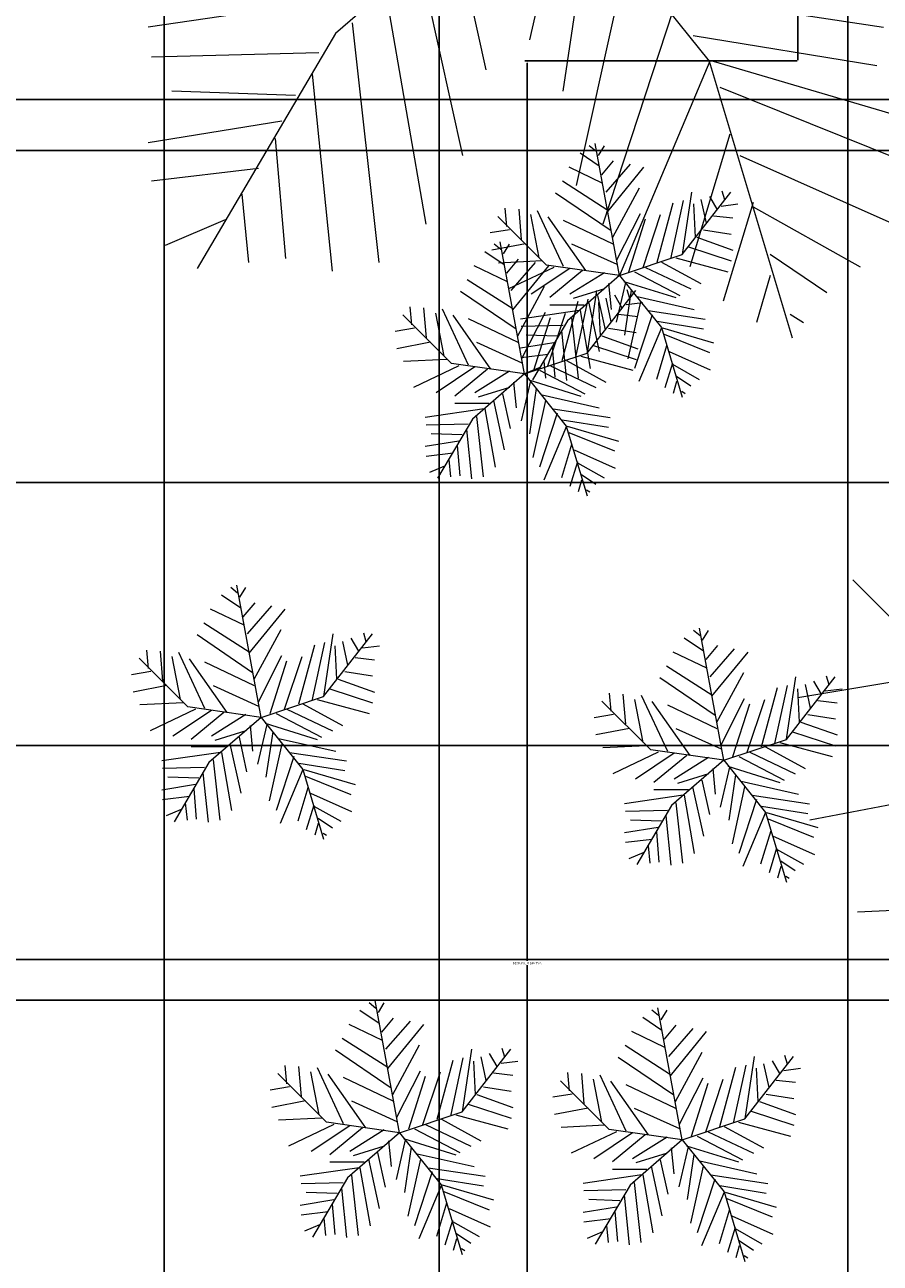
# Model space of a CAD drawing. Units: inches. Extents: x 818 to 1898, y 976 to 2364.
# Tile 12 of 96: x 1002 to 1071, y 1773 to 1873. Entities that reach past the tile are written whole.
import ezdxf

# ---------------------------------------------------------------- set-up
doc = ezdxf.new("R2010")
doc.units = ezdxf.units.IN
doc.header["$LTSCALE"] = 5
doc.header["$MEASUREMENT"] = 0
doc.layers.add('A-ANNO-DIMS', color=2, linetype='Continuous', lineweight=18)
doc.layers.add('L-PLNT', color=116, linetype='Continuous', lineweight=13, true_color=0x136734)
doc.styles.get("Standard").update_dxf_attribs({"font": 'arial.ttf'})
doc.dimstyles.get("Standard").update_dxf_attribs({"dimtxt": 0.18, "dimasz": 0.18, "dimexe": 0.18, "dimexo": 0.0625, "dimgap": 0.09, "dimtad": 0, "dimtih": 1, "dimtoh": 1, "dimdec": 4, "dimzin": 0, "dimdsep": 46, "dimtxsty": 'Standard', "dimcen": 0.09, "dimadec": 0, "dimazin": 0, "dimtfac": 1, "dimtdec": 4, "dimtofl": 0, "dimtmove": 0, "dimatfit": 3, "dimfxl": 1, "dimtolj": 1, "dimtzin": 0, "dimarcsym": 0})

# ---------------------------------------------------------------- blocks, each defined once
blk = doc.blocks.new('SHRUB-ACCENT')
for p, q in [((8.533, 19.844), (7.992, 20.278)), ((10.438, 9.815), (8.475, 20.472)), ((8.737, 19.496), (9.211, 20.278)), ((8.804, 18.628), (7.247, 19.67)), ((9.008, 17.934), (9.956, 19.062)), ((9.075, 17.239), (6.366, 18.541)), ((9.346, 16.544), (11.31, 18.802)), ((9.482, 14.981), (12.394, 18.541)), ((9.482, 15.068), (5.824, 17.413)), ((9.753, 13.419), (5.283, 16.458)), ((9.888, 12.898), (12.055, 16.892)), ((15.486, 11.498), (19.412, 16.546)), ((15.509, 11.509), (16.254, 16.544)), ((17.677, 16.197), (18.286, 15.155)), ((18.693, 16.631), (18.896, 15.937)), ((1.354, 13.766), (1.219, 15.242)), ((2.303, 15.155), (2.506, 12.724)), ((3.793, 15.068), (5.892, 10.553)), ((13.478, 10.901), (14.764, 15.676)), ((14.561, 11.161), (15.577, 15.85)), ((16.39, 15.589), (16.525, 12.898)), ((16.999, 15.937), (17.406, 14.026)), ((18.625, 15.416), (19.979, 15.589)), ((4.549, 10.657), (0.623, 14.583)), ((3.251, 14.721), (3.928, 11.248)), ((7.721, 10.206), (4.673, 14.547)), ((5.892, 14.287), (9.888, 12.377)), ((10.227, 11.074), (12.123, 14.808)), ((11.175, 10.119), (12.529, 14.374)), ((12.326, 10.467), (13.748, 14.721)), ((18.015, 14.634), (19.573, 14.461)), ((1.558, 13.505), (0, 13.245)), ((17.203, 13.505), (19.437, 13.158)), ((2.845, 12.377), (0.136, 11.856)), ((6.569, 12.377), (10.227, 10.727)), ((15.983, 12.116), (19.437, 10.988)), ((16.661, 12.898), (19.573, 11.856)), ((4.199, 10.988), (0.677, 10.814)), ((10.438, 9.815), (15.486, 11.498)), ((14.968, 11.248), (19.166, 10.119)), ((5.147, 10.467), (1.49, 8.73)), ((6.434, 10.38), (3.319, 8.296)), ((10.438, 9.815), (4.549, 10.657)), ((7.45, 10.206), (4.809, 8.035)), ((9.211, 10.033), (6.434, 8.296)), ((11.649, 10.119), (15.306, 8.209)), ((12.529, 10.467), (16.187, 8.73)), ((13.816, 10.901), (16.999, 9.164)), ((10.438, 9.815), (6.231, 6.17)), ((9.549, 9.164), (9.753, 7.08)), ((10.904, 9.251), (10.159, 6.039)), ((10.438, 9.815), (13.803, 5.609)), ((10.769, 9.338), (14.968, 8.035)), ((9.211, 8.73), (6.705, 7.949)), ((8.669, 8.209), (9.278, 5.431)), ((11.378, 8.643), (10.836, 4.997)), ((11.852, 8.122), (16.457, 7.08)), ((7.179, 6.994), (2.438, 6.299)), ((7.585, 7.428), (4.809, 7.428)), ((7.247, 6.994), (8.06, 2.305)), ((7.924, 7.688), (8.804, 3.694)), ((12.123, 7.688), (11.107, 3.086)), ((12.733, 6.994), (17.338, 6.299)), ((6.231, 6.17), (3.427, 1.402)), ((6.569, 6.386), (7.111, 1.524)), ((13.071, 6.646), (11.649, 2.305)), ((13.478, 6.125), (17.203, 5.517)), ((5.892, 5.778), (2.506, 5.691)), ((5.418, 4.91), (2.912, 4.997)), ((5.757, 5.344), (6.163, 1.35)), ((13.816, 5.604), (11.988, 1.263)), ((13.803, 5.609), (15.486, 0)), ((13.884, 5.604), (18.015, 4.389)), ((14.019, 5.083), (17.677, 3.607)), ((5.147, 4.389), (2.438, 3.955)), ((5.012, 4.041), (5.215, 1.61)), ((14.223, 4.128), (13.41, 1.437)), ((4.673, 3.434), (2.506, 3.173)), ((14.426, 3.694), (17.744, 2.218)), ((3.996, 2.392), (2.777, 1.871)), ((4.334, 2.913), (4.47, 1.524)), ((14.697, 2.739), (14.087, 0.742)), ((14.697, 2.652), (16.864, 1.437)), ((15.035, 1.263), (14.764, 0.308)), ((15.035, 1.697), (16.187, 0.916)), ((15.442, 0.482), (15.712, 0.308))]:
    blk.add_line(p, q)
blk = doc.blocks.new('PALM-BORDER')
for p, q in [((41.528, 39.051), (33.718, 81.449)), ((33.951, 78.95), (31.796, 80.677)), ((34.76, 77.568), (36.646, 80.677)), ((35.029, 74.114), (28.831, 78.259)), ((35.838, 71.35), (39.61, 75.841)), ((37.185, 65.823), (44.999, 74.805)), ((36.107, 68.586), (25.329, 73.768)), ((37.724, 59.605), (49.31, 73.768)), ((37.724, 59.95), (23.173, 69.277)), ((39.34, 51.314), (47.963, 67.205)), ((74.37, 66.168), (75.178, 63.405)), ((38.802, 53.387), (21.018, 65.477)), ((61.611, 45.746), (77.231, 65.829)), ((61.706, 45.787), (64.67, 65.823)), ((70.328, 64.441), (72.753, 60.296)), ((57.933, 44.405), (61.975, 63.06)), ((67.633, 63.405), (69.25, 55.805)), ((53.622, 43.369), (58.741, 62.369)), ((65.208, 62.023), (65.748, 51.314)), ((74.101, 61.332), (79.49, 62.023)), ((5.389, 54.769), (4.85, 60.641)), ((9.162, 60.296), (9.97, 50.624)), ((15.089, 59.95), (23.442, 41.987)), ((18.097, 42.398), (2.477, 58.019)), ((12.934, 58.568), (15.629, 44.751)), ((40.688, 44.06), (48.233, 58.914)), ((49.041, 41.642), (54.699, 58.568)), ((71.675, 58.223), (77.873, 57.532)), ((30.718, 40.606), (18.593, 57.877)), ((44.46, 40.26), (49.849, 57.186)), ((23.442, 56.841), (39.34, 49.242)), ((6.198, 53.732), (0, 52.696)), ((68.442, 53.732), (77.333, 52.351)), ((66.286, 51.314), (77.873, 47.169)), ((11.317, 49.242), (0.539, 47.169)), ((26.137, 49.242), (40.688, 42.678)), ((63.591, 48.205), (77.333, 43.714)), ((41.528, 39.051), (61.611, 45.746)), ((59.55, 44.751), (76.256, 40.26)), ((16.706, 43.714), (2.695, 43.023)), ((54.969, 43.369), (67.633, 36.46)), ((41.528, 39.051), (18.097, 42.398)), ((20.478, 41.642), (5.928, 34.733)), ((25.598, 41.296), (13.204, 33.005)), ((49.849, 41.642), (64.4, 34.733)), ((29.64, 40.606), (19.131, 31.969)), ((46.346, 40.26), (60.897, 32.66)), ((41.528, 39.051), (24.792, 24.547)), ((36.646, 39.915), (25.598, 33.005)), ((41.528, 39.051), (54.917, 22.315)), ((42.844, 37.151), (59.55, 31.969)), ((37.993, 36.46), (38.802, 28.17)), ((43.382, 36.806), (40.419, 24.024)), ((36.646, 34.733), (26.676, 31.624)), ((45.268, 34.387), (43.113, 19.879)), ((34.49, 32.66), (36.915, 21.606)), ((47.155, 32.315), (65.477, 28.17)), ((31.526, 30.588), (35.029, 14.698)), ((48.233, 30.588), (44.191, 12.279)), ((30.179, 29.551), (19.131, 29.551)), ((28.562, 27.824), (9.7, 25.061)), ((28.831, 27.824), (32.066, 9.17)), ((50.658, 27.824), (68.98, 25.061)), ((52.005, 26.443), (46.346, 9.17)), ((26.137, 25.406), (28.293, 6.061)), ((24.792, 24.547), (13.634, 5.579)), ((53.622, 24.37), (68.442, 21.951)), ((23.442, 22.987), (9.97, 22.642)), ((54.969, 22.297), (47.693, 5.025)), ((54.917, 22.315), (61.611, 0)), ((55.239, 22.297), (71.675, 17.461)), ((22.904, 21.26), (24.52, 5.37)), ((55.777, 20.224), (70.328, 14.352)), ((21.557, 19.533), (11.587, 19.879)), ((20.478, 17.461), (9.7, 15.734)), ((19.94, 16.079), (20.748, 6.407)), ((56.586, 16.425), (53.352, 5.716)), ((57.394, 14.698), (70.597, 8.825)), ((18.593, 13.661), (9.97, 12.625)), ((17.245, 11.588), (17.784, 6.061)), ((58.472, 10.897), (56.047, 2.952)), ((58.472, 10.552), (67.095, 5.716)), ((15.898, 9.515), (11.047, 7.443)), ((59.819, 6.752), (64.4, 3.643)), ((59.819, 5.025), (58.741, 1.225)), ((61.436, 1.916), (62.513, 1.225))]:
    blk.add_line(p, q)
blk = doc.blocks.new('PALM-DECK')
for p, q in [((32.333, 75.749), (4.425, 103.656)), ((11.073, 95.998), (0, 94.146)), ((20.22, 87.975), (0.964, 84.271)), ((29.848, 78.1), (4.815, 76.865))]:
    blk.add_line(p, q)
blk = doc.blocks.new('*D28')
at = {"layer": 'A-ANNO-DIMS', "color": 0, "lineweight": -2, "ltscale": 5, "transparency": 16777216}
for p, q in [((1064.248, 1870.181), (1042.302, 1870.181)), ((1042.482, 1870.001), (1042.482, 1797.606)), ((1042.482, 1724.844), (1042.482, 1797.24)), ((1064.248, 1724.664), (1042.302, 1724.664))]:
    blk.add_line(p, q, dxfattribs=at)
at = {"layer": 'A-ANNO-DIMS', "color": 0, "ltscale": 5, "transparency": 16777216}
for points in [[(1042.452, 1870.001), (1042.512, 1870.001), (1042.482, 1870.181)], [(1042.452, 1724.844), (1042.512, 1724.844), (1042.482, 1724.664)]]:
    blk.add_solid(points, dxfattribs=at)
at = {"layer": 'Defpoints', "color": 0, "ltscale": 5, "transparency": 16777216}
for p in [(1042.482, 1870.181), (1064.31, 1870.181), (1064.31, 1724.664)]:
    blk.add_point(p, dxfattribs=at)
at = {"layer": 'A-ANNO-DIMS', "color": 0, "ltscale": 5, "transparency": 16777216, "insert": (1042.482, 1797.423), "char_height": 0.18, "attachment_point": 5}
blk.add_mtext('\\A1;DECK PALM 146 TYP.', dxfattribs=at)
blk = doc.blocks.new('*D29')
at = {"layer": 'A-ANNO-DIMS', "color": 0, "lineweight": -2, "ltscale": 5, "transparency": 16777216}
for p, q in [((1064.31, 1870.244), (1064.31, 1892.189)), ((1064.49, 1892.009), (1134.729, 1892.009)), ((1206.147, 1892.009), (1135.908, 1892.009)), ((1206.327, 1870.244), (1206.327, 1892.189))]:
    blk.add_line(p, q, dxfattribs=at)
at = {"layer": 'A-ANNO-DIMS', "color": 0, "ltscale": 5, "transparency": 16777216}
for points in [[(1064.49, 1892.039), (1064.49, 1891.979), (1064.31, 1892.009)], [(1206.147, 1892.039), (1206.147, 1891.979), (1206.327, 1892.009)]]:
    blk.add_solid(points, dxfattribs=at)
at = {"layer": 'Defpoints', "color": 0, "ltscale": 5, "transparency": 16777216}
for p in [(1206.327, 1892.009), (1064.31, 1870.181), (1206.327, 1870.181)]:
    blk.add_point(p, dxfattribs=at)
at = {"layer": 'A-ANNO-DIMS', "color": 0, "ltscale": 5, "transparency": 16777216, "insert": (1135.319, 1892.009), "char_height": 0.18, "attachment_point": 5}
blk.add_mtext('\\A1;142 TYP.', dxfattribs=at)
blk = doc.blocks.new('*D59')
at = {"layer": 'A-ANNO-DIMS', "color": 0, "lineweight": -2, "ltscale": 5, "transparency": 16777216}
for p, q in [((1251.643, 2300.393), (818.026, 2300.393)), ((818.206, 2300.213), (818.206, 1669.95)), ((818.206, 1039.323), (818.206, 1669.586)), ((896.051, 1039.143), (818.026, 1039.143))]:
    blk.add_line(p, q, dxfattribs=at)
at = {"layer": 'A-ANNO-DIMS', "color": 0, "ltscale": 5, "transparency": 16777216}
for points in [[(818.176, 2300.213), (818.236, 2300.213), (818.206, 2300.393)], [(818.176, 1039.323), (818.236, 1039.323), (818.206, 1039.143)]]:
    blk.add_solid(points, dxfattribs=at)
at = {"layer": 'Defpoints', "color": 0, "ltscale": 5, "transparency": 16777216}
for p in [(818.206, 2300.393), (1251.706, 2300.393), (896.114, 1039.143)]:
    blk.add_point(p, dxfattribs=at)
at = {"layer": 'A-ANNO-DIMS', "color": 0, "ltscale": 5, "transparency": 16777216, "insert": (818.206, 1669.768), "char_height": 0.18, "attachment_point": 5}
blk.add_mtext('\\A1;1261.2', dxfattribs=at)
blk = doc.blocks.new('*D79')
at = {"layer": 'A-ANNO-DIMS', "color": 0, "lineweight": -2, "ltscale": 5, "transparency": 16777216}
for p, q in [((992.725, 1203.027), (992.725, 2363.873)), ((992.905, 2363.693), (1032.007, 2363.693)), ((1071.545, 2363.693), (1032.444, 2363.693)), ((1071.725, 1203.027), (1071.725, 2363.873))]:
    blk.add_line(p, q, dxfattribs=at)
at = {"layer": 'A-ANNO-DIMS', "color": 0, "ltscale": 5, "transparency": 16777216}
for points in [[(992.905, 2363.723), (992.905, 2363.663), (992.725, 2363.693)], [(1071.545, 2363.723), (1071.545, 2363.663), (1071.725, 2363.693)]]:
    blk.add_solid(points, dxfattribs=at)
at = {"layer": 'Defpoints', "color": 0, "ltscale": 5, "transparency": 16777216}
for p in [(1071.725, 2363.693), (992.725, 1202.964), (1071.725, 1202.964)]:
    blk.add_point(p, dxfattribs=at)
at = {"layer": 'A-ANNO-DIMS', "color": 0, "ltscale": 5, "transparency": 16777216, "insert": (1032.225, 2363.693), "char_height": 0.18, "attachment_point": 5}
blk.add_mtext('\\A1;79', dxfattribs=at)
blk = doc.blocks.new('*D91')
at = {"layer": 'A-ANNO-DIMS', "color": 0, "lineweight": -2, "ltscale": 5, "transparency": 16777216}
for p, q in [((959.174, 1071.118), (959.174, 2363.873)), ((959.354, 2363.693), (985.802, 2363.693)), ((1013.038, 2363.693), (986.589, 2363.693)), ((1013.218, 1071.118), (1013.218, 2363.873))]:
    blk.add_line(p, q, dxfattribs=at)
at = {"layer": 'A-ANNO-DIMS', "color": 0, "ltscale": 5, "transparency": 16777216}
for points in [[(959.354, 2363.723), (959.354, 2363.663), (959.174, 2363.693)], [(1013.038, 2363.723), (1013.038, 2363.663), (1013.218, 2363.693)]]:
    blk.add_solid(points, dxfattribs=at)
at = {"layer": 'Defpoints', "color": 0, "ltscale": 5, "transparency": 16777216}
for p in [(1013.218, 2363.693), (959.174, 1071.055), (1013.218, 1071.055)]:
    blk.add_point(p, dxfattribs=at)
at = {"layer": 'A-ANNO-DIMS', "color": 0, "ltscale": 5, "transparency": 16777216, "insert": (986.196, 2363.693), "char_height": 0.18, "attachment_point": 5}
blk.add_mtext('\\A1;54.04', dxfattribs=at)
blk = doc.blocks.new('*D92')
at = {"layer": 'A-ANNO-DIMS', "color": 0, "lineweight": -2, "ltscale": 5, "transparency": 16777216}
for p, q in [((1013.218, 1071.118), (1013.218, 2363.873)), ((1013.398, 2363.693), (1040.385, 2363.693)), ((1068.158, 2363.693), (1041.17, 2363.693)), ((1068.338, 1071.118), (1068.338, 2363.873))]:
    blk.add_line(p, q, dxfattribs=at)
at = {"layer": 'A-ANNO-DIMS', "color": 0, "ltscale": 5, "transparency": 16777216}
for points in [[(1013.398, 2363.723), (1013.398, 2363.663), (1013.218, 2363.693)], [(1068.158, 2363.723), (1068.158, 2363.663), (1068.338, 2363.693)]]:
    blk.add_solid(points, dxfattribs=at)
at = {"layer": 'Defpoints', "color": 0, "ltscale": 5, "transparency": 16777216}
for p in [(1068.338, 2363.693), (1013.218, 1071.055), (1068.338, 1071.055)]:
    blk.add_point(p, dxfattribs=at)
at = {"layer": 'A-ANNO-DIMS', "color": 0, "ltscale": 5, "transparency": 16777216, "insert": (1040.778, 2363.693), "char_height": 0.18, "attachment_point": 5}
blk.add_mtext('\\A1;55.12', dxfattribs=at)
blk = doc.blocks.new('*D93')
at = {"layer": 'A-ANNO-DIMS', "color": 0, "lineweight": -2, "ltscale": 5, "transparency": 16777216}
for p, q in [((1068.338, 1071.118), (1068.338, 2363.873)), ((1068.518, 2363.693), (1094.157, 2363.693)), ((1120.582, 2363.693), (1094.942, 2363.693)), ((1120.762, 1071.118), (1120.762, 2363.873))]:
    blk.add_line(p, q, dxfattribs=at)
at = {"layer": 'A-ANNO-DIMS', "color": 0, "ltscale": 5, "transparency": 16777216}
for points in [[(1068.518, 2363.723), (1068.518, 2363.663), (1068.338, 2363.693)], [(1120.582, 2363.723), (1120.582, 2363.663), (1120.762, 2363.693)]]:
    blk.add_solid(points, dxfattribs=at)
at = {"layer": 'Defpoints', "color": 0, "ltscale": 5, "transparency": 16777216}
for p in [(1120.762, 2363.693), (1068.338, 1071.055), (1120.762, 1071.055)]:
    blk.add_point(p, dxfattribs=at)
at = {"layer": 'A-ANNO-DIMS', "color": 0, "ltscale": 5, "transparency": 16777216, "insert": (1094.55, 2363.693), "char_height": 0.18, "attachment_point": 5}
blk.add_mtext('\\A1;52.42', dxfattribs=at)
blk = doc.blocks.new('*D120')
at = {"layer": 'A-ANNO-DIMS', "color": 0, "lineweight": -2, "ltscale": 5, "transparency": 16777216}
for p, q in [((1766.29, 1797.717), (818.026, 1797.717)), ((818.206, 1797.537), (818.206, 1757.534)), ((818.206, 1717.167), (818.206, 1757.17)), ((1766.29, 1716.987), (818.026, 1716.987))]:
    blk.add_line(p, q, dxfattribs=at)
at = {"layer": 'A-ANNO-DIMS', "color": 0, "ltscale": 5, "transparency": 16777216}
for points in [[(818.176, 1797.537), (818.236, 1797.537), (818.206, 1797.717)], [(818.176, 1717.167), (818.236, 1717.167), (818.206, 1716.987)]]:
    blk.add_solid(points, dxfattribs=at)
at = {"layer": 'Defpoints', "color": 0, "ltscale": 5, "transparency": 16777216}
for p in [(818.206, 1797.717), (1766.352, 1797.717), (1766.352, 1716.987)]:
    blk.add_point(p, dxfattribs=at)
at = {"layer": 'A-ANNO-DIMS', "color": 0, "ltscale": 5, "transparency": 16777216, "insert": (818.206, 1757.352), "char_height": 0.18, "attachment_point": 5}
blk.add_mtext('\\A1;80.73', dxfattribs=at)
blk = doc.blocks.new('*D121')
at = {"layer": 'A-ANNO-DIMS', "color": 0, "lineweight": -2, "ltscale": 5, "transparency": 16777216}
for p, q in [((1766.29, 1884.203), (818.026, 1884.203)), ((818.206, 1884.023), (818.206, 1841.142)), ((818.206, 1797.897), (818.206, 1840.778)), ((1766.29, 1797.717), (818.026, 1797.717))]:
    blk.add_line(p, q, dxfattribs=at)
at = {"layer": 'A-ANNO-DIMS', "color": 0, "ltscale": 5, "transparency": 16777216}
for points in [[(818.176, 1884.023), (818.236, 1884.023), (818.206, 1884.203)], [(818.176, 1797.897), (818.236, 1797.897), (818.206, 1797.717)]]:
    blk.add_solid(points, dxfattribs=at)
at = {"layer": 'Defpoints', "color": 0, "ltscale": 5, "transparency": 16777216}
for p in [(818.206, 1884.203), (1766.352, 1884.203), (1766.352, 1797.717)]:
    blk.add_point(p, dxfattribs=at)
at = {"layer": 'A-ANNO-DIMS', "color": 0, "ltscale": 5, "transparency": 16777216, "insert": (818.206, 1840.96), "char_height": 0.18, "attachment_point": 5}
blk.add_mtext('\\A1;86.49', dxfattribs=at)
blk = doc.blocks.new('*D124')
at = {"layer": 'A-ANNO-DIMS', "color": 0, "lineweight": -2, "ltscale": 5, "transparency": 16777216}
for p, q in [((1131.703, 1974.573), (818.026, 1974.573)), ((818.206, 1974.393), (818.206, 1884.685)), ((818.206, 1794.613), (818.206, 1884.321)), ((1138.442, 1794.433), (818.026, 1794.433))]:
    blk.add_line(p, q, dxfattribs=at)
at = {"layer": 'A-ANNO-DIMS', "color": 0, "ltscale": 5, "transparency": 16777216}
for points in [[(818.176, 1974.393), (818.236, 1974.393), (818.206, 1974.573)], [(818.176, 1794.613), (818.236, 1794.613), (818.206, 1794.433)]]:
    blk.add_solid(points, dxfattribs=at)
at = {"layer": 'Defpoints', "color": 0, "ltscale": 5, "transparency": 16777216}
for p in [(818.206, 1974.573), (1131.765, 1974.573), (1138.504, 1794.433)]:
    blk.add_point(p, dxfattribs=at)
at = {"layer": 'A-ANNO-DIMS', "color": 0, "ltscale": 5, "transparency": 16777216, "insert": (818.206, 1884.503), "char_height": 0.18, "attachment_point": 5}
blk.add_mtext('\\A1;180.14', dxfattribs=at)
blk = doc.blocks.new('*D126')
at = {"layer": 'A-ANNO-DIMS', "color": 0, "lineweight": -2, "ltscale": 5, "transparency": 16777216}
for p, q in [((1035.377, 1252.087), (1035.377, 2363.873)), ((1035.557, 2363.693), (1075.406, 2363.693)), ((1116.008, 2363.693), (1076.159, 2363.693)), ((1116.188, 1236.027), (1116.188, 2363.873))]:
    blk.add_line(p, q, dxfattribs=at)
at = {"layer": 'A-ANNO-DIMS', "color": 0, "ltscale": 5, "transparency": 16777216}
for points in [[(1035.557, 2363.723), (1035.557, 2363.663), (1035.377, 2363.693)], [(1116.008, 2363.723), (1116.008, 2363.663), (1116.188, 2363.693)]]:
    blk.add_solid(points, dxfattribs=at)
at = {"layer": 'Defpoints', "color": 0, "ltscale": 5, "transparency": 16777216}
for p in [(1035.377, 2363.693), (1035.377, 1252.024), (1116.188, 1235.964)]:
    blk.add_point(p, dxfattribs=at)
at = {"layer": 'A-ANNO-DIMS', "color": 0, "ltscale": 5, "transparency": 16777216, "insert": (1075.782, 2363.693), "char_height": 0.18, "attachment_point": 5}
blk.add_mtext('\\A1;80.81', dxfattribs=at)
blk = doc.blocks.new('*D131')
at = {"layer": 'A-ANNO-DIMS', "color": 0, "lineweight": -2, "ltscale": 5, "transparency": 16777216}
for p, q in [((1043.706, 1886.902), (818.026, 1886.902)), ((818.206, 1886.722), (818.206, 1805.948)), ((818.206, 1724.81), (818.206, 1805.584)), ((1044.784, 1724.63), (818.026, 1724.63))]:
    blk.add_line(p, q, dxfattribs=at)
at = {"layer": 'A-ANNO-DIMS', "color": 0, "ltscale": 5, "transparency": 16777216}
for points in [[(818.176, 1886.722), (818.236, 1886.722), (818.206, 1886.902)], [(818.176, 1724.81), (818.236, 1724.81), (818.206, 1724.63)]]:
    blk.add_solid(points, dxfattribs=at)
at = {"layer": 'Defpoints', "color": 0, "ltscale": 5, "transparency": 16777216}
for p in [(818.206, 1886.902), (1043.769, 1886.902), (1044.846, 1724.63)]:
    blk.add_point(p, dxfattribs=at)
at = {"layer": 'A-ANNO-DIMS', "color": 0, "ltscale": 5, "transparency": 16777216, "insert": (818.206, 1805.766), "char_height": 0.18, "attachment_point": 5}
blk.add_mtext('\\A1;162.27', dxfattribs=at)
blk = doc.blocks.new('*D162')
at = {"layer": 'A-ANNO-DIMS', "color": 0, "lineweight": -2, "ltscale": 5, "transparency": 16777216}
for p, q in [((1429.163, 1876.078), (818.026, 1876.078)), ((818.206, 1875.898), (818.206, 1871.76)), ((818.206, 1867.258), (818.206, 1871.396)), ((1429.163, 1867.078), (818.026, 1867.078))]:
    blk.add_line(p, q, dxfattribs=at)
at = {"layer": 'A-ANNO-DIMS', "color": 0, "ltscale": 5, "transparency": 16777216}
for points in [[(818.176, 1875.898), (818.236, 1875.898), (818.206, 1876.078)], [(818.176, 1867.258), (818.236, 1867.258), (818.206, 1867.078)]]:
    blk.add_solid(points, dxfattribs=at)
at = {"layer": 'Defpoints', "color": 0, "ltscale": 5, "transparency": 16777216}
for p in [(1429.225, 1876.078), (818.206, 1867.078), (1429.225, 1867.078)]:
    blk.add_point(p, dxfattribs=at)
at = {"layer": 'A-ANNO-DIMS', "color": 0, "ltscale": 5, "transparency": 16777216, "insert": (818.206, 1871.578), "char_height": 0.18, "attachment_point": 5}
blk.add_mtext('\\A1;9', dxfattribs=at)
blk = doc.blocks.new('*D215')
at = {"layer": 'A-ANNO-DIMS', "color": 0, "lineweight": -2, "ltscale": 5, "transparency": 16777216}
for p, q in [((1590.663, 1876.078), (818.026, 1876.078)), ((818.206, 1875.898), (818.206, 1781.76)), ((818.206, 1687.258), (818.206, 1781.396)), ((1511.663, 1687.078), (818.026, 1687.078))]:
    blk.add_line(p, q, dxfattribs=at)
at = {"layer": 'A-ANNO-DIMS', "color": 0, "ltscale": 5, "transparency": 16777216}
for points in [[(818.176, 1875.898), (818.236, 1875.898), (818.206, 1876.078)], [(818.176, 1687.258), (818.236, 1687.258), (818.206, 1687.078)]]:
    blk.add_solid(points, dxfattribs=at)
at = {"layer": 'Defpoints', "color": 0, "ltscale": 5, "transparency": 16777216}
for p in [(818.206, 1876.078), (1590.725, 1876.078), (1511.725, 1687.078)]:
    blk.add_point(p, dxfattribs=at)
at = {"layer": 'A-ANNO-DIMS', "color": 0, "ltscale": 5, "transparency": 16777216, "insert": (818.206, 1781.578), "char_height": 0.18, "attachment_point": 5}
blk.add_mtext('\\A1;189', dxfattribs=at)
blk = doc.blocks.new('*D227')
at = {"layer": 'A-ANNO-DIMS', "color": 0, "lineweight": -2, "ltscale": 5, "transparency": 16777216}
for p, q in [((1595.663, 1867.078), (818.026, 1867.078)), ((818.206, 1866.898), (818.206, 1851.813)), ((818.206, 1836.364), (818.206, 1851.449)), ((1594.663, 1836.184), (818.026, 1836.184))]:
    blk.add_line(p, q, dxfattribs=at)
at = {"layer": 'A-ANNO-DIMS', "color": 0, "ltscale": 5, "transparency": 16777216}
for points in [[(818.176, 1866.898), (818.236, 1866.898), (818.206, 1867.078)], [(818.176, 1836.364), (818.236, 1836.364), (818.206, 1836.184)]]:
    blk.add_solid(points, dxfattribs=at)
at = {"layer": 'Defpoints', "color": 0, "ltscale": 5, "transparency": 16777216}
for p in [(818.206, 1867.078), (1595.725, 1867.078), (1594.725, 1836.184)]:
    blk.add_point(p, dxfattribs=at)
at = {"layer": 'A-ANNO-DIMS', "color": 0, "ltscale": 5, "transparency": 16777216, "insert": (818.206, 1851.631), "char_height": 0.18, "attachment_point": 5}
blk.add_mtext('\\A1;30.894', dxfattribs=at)
blk = doc.blocks.new('*D247')
at = {"layer": 'A-ANNO-DIMS', "color": 0, "lineweight": -2, "ltscale": 5, "transparency": 16777216}
for p, q in [((1258.663, 1862.965), (818.026, 1862.965)), ((818.206, 1862.785), (818.206, 1839.147)), ((818.206, 1815.145), (818.206, 1838.783)), ((1258.663, 1814.965), (818.026, 1814.965))]:
    blk.add_line(p, q, dxfattribs=at)
at = {"layer": 'A-ANNO-DIMS', "color": 0, "ltscale": 5, "transparency": 16777216}
for points in [[(818.176, 1862.785), (818.236, 1862.785), (818.206, 1862.965)], [(818.176, 1815.145), (818.236, 1815.145), (818.206, 1814.965)]]:
    blk.add_solid(points, dxfattribs=at)
at = {"layer": 'Defpoints', "color": 0, "ltscale": 5, "transparency": 16777216}
for p in [(818.206, 1862.965), (1258.725, 1862.965), (1258.725, 1814.965)]:
    blk.add_point(p, dxfattribs=at)
at = {"layer": 'A-ANNO-DIMS', "color": 0, "ltscale": 5, "transparency": 16777216, "insert": (818.206, 1838.965), "char_height": 0.18, "attachment_point": 5}
blk.add_mtext('\\A1;48', dxfattribs=at)
blk = doc.blocks.new('*D249')
at = {"layer": 'A-ANNO-DIMS', "color": 0, "lineweight": -2, "ltscale": 5, "transparency": 16777216}
for p, q in [((1258.663, 1814.965), (818.026, 1814.965)), ((818.206, 1814.785), (818.206, 1785.331)), ((818.206, 1755.512), (818.206, 1784.967)), ((1258.663, 1755.332), (818.026, 1755.332))]:
    blk.add_line(p, q, dxfattribs=at)
at = {"layer": 'A-ANNO-DIMS', "color": 0, "ltscale": 5, "transparency": 16777216}
for points in [[(818.176, 1814.785), (818.236, 1814.785), (818.206, 1814.965)], [(818.176, 1755.512), (818.236, 1755.512), (818.206, 1755.332)]]:
    blk.add_solid(points, dxfattribs=at)
at = {"layer": 'Defpoints', "color": 0, "ltscale": 5, "transparency": 16777216}
for p in [(818.206, 1814.965), (1258.725, 1814.965), (1258.725, 1755.332)]:
    blk.add_point(p, dxfattribs=at)
at = {"layer": 'A-ANNO-DIMS', "color": 0, "ltscale": 5, "transparency": 16777216, "insert": (818.206, 1785.149), "char_height": 0.18, "attachment_point": 5}
blk.add_mtext('\\A1;59.63', dxfattribs=at)

msp = doc.modelspace()

# ---------------------------------------------------------------- block references
at = {"layer": 'L-PLNT'}
for name, p in [('PALM-BORDER', (1002.2407, 1847.8507)), ('PALM-DECK', (1064.31, 1724.664)), ('SHRUB-ACCENT', (1039.4963, 1843.0601)), ('SHRUB-ACCENT', (1031.8351, 1835.1155)), ('SHRUB-ACCENT', (1010.5905, 1807.4231)), ('SHRUB-ACCENT', (1047.8927, 1803.9599)), ('SHRUB-ACCENT', (1021.7558, 1773.927)), ('SHRUB-ACCENT', (1044.5479, 1773.3498))]:
    msp.add_blockref(name, p, dxfattribs=at)

# ---------------------------------------------------------------- dimensions: what is measured, and where the dimension line sits
at = {"layer": 'A-ANNO-DIMS', "ltscale": 5}
for base, p1, p2, override, picture, middle in [((1013.2176, 2363.6929), (959.1737, 1071.0552), (1013.2176, 1071.0552), {"dimdec": 2, "dimlfac": 1, "dimrnd": 0, "dimzin": 0, "dimdsep": 46, "dimlunit": 2}, '*D91', (986.1956, 2363.6929)), ((1071.7251, 2363.6929), (992.7251, 1202.9642), (1071.7251, 1202.9642), {"dimdec": 0, "dimlfac": 1, "dimrnd": 0, "dimzin": 0, "dimdsep": 46, "dimlunit": 2}, '*D79', (1032.2251, 2363.6929)), ((1068.3377, 2363.6929), (1013.2176, 1071.0552), (1068.3377, 1071.0552), {"dimdec": 2, "dimlfac": 1, "dimrnd": 0, "dimzin": 0, "dimdsep": 46, "dimlunit": 2}, '*D92', (1040.7776, 2363.6929)), ((1035.3768, 2363.6929), (1116.1882, 1235.9642), (1035.3768, 1252.0242), {"dimdec": 2, "dimlfac": 1, "dimrnd": 0, "dimzin": 0, "dimdsep": 46, "dimlunit": 2}, '*D126', (1075.7825, 2363.6929)), ((1120.7618, 2363.6929), (1068.3377, 1071.0552), (1120.7618, 1071.0552), {"dimdec": 2, "dimlfac": 1, "dimrnd": 0, "dimzin": 0, "dimdsep": 46, "dimlunit": 2}, '*D93', (1094.5497, 2363.6929))]:
    dim = msp.add_linear_dim(base=base, p1=p1, p2=p2, dimstyle='Standard', override=override, dxfattribs=at)
    dim.commit()
    dim.dimension.update_dxf_attribs({"geometry": picture, "text_midpoint": middle})
for base, p1, p2, override, picture, middle in [((818.2059, 2300.3929), (896.1138, 1039.1433), (1251.7057, 2300.3929), {"dimdec": 1, "dimlfac": 1, "dimrnd": 0, "dimzin": 0, "dimdsep": 46, "dimlunit": 2}, '*D59', (818.2059, 1669.7681)), ((818.2059, 1974.5735), (1138.5041, 1794.4325), (1131.7651, 1974.5735), {"dimdec": 2, "dimlfac": 1, "dimrnd": 0, "dimzin": 0, "dimdsep": 46, "dimlunit": 2}, '*D124', (818.2059, 1884.503)), ((818.2059, 1886.9018), (1044.8463, 1724.63), (1043.7685, 1886.9018), {"dimdec": 2, "dimlfac": 1, "dimrnd": 0, "dimzin": 0, "dimdsep": 46, "dimlunit": 2}, '*D131', (818.2059, 1805.7659)), ((818.2059, 1884.2031), (1766.3524, 1797.7165), (1766.3524, 1884.2031), {"dimdec": 2, "dimlfac": 1, "dimrnd": 0, "dimzin": 0, "dimdsep": 46, "dimlunit": 2}, '*D121', (818.2059, 1840.9598)), ((818.2059, 1876.0782), (1511.7251, 1687.0782), (1590.7251, 1876.0782), {"dimdec": 0, "dimlfac": 1, "dimrnd": 0, "dimzin": 0, "dimdsep": 46, "dimlunit": 2}, '*D215', (818.2059, 1781.5782)), ((818.2059, 1867.0782), (1429.2251, 1876.0782), (1429.2251, 1867.0782), {"dimdec": 0, "dimlfac": 1, "dimrnd": 0, "dimzin": 0, "dimdsep": 46, "dimlunit": 2}, '*D162', (818.2059, 1871.5782)), ((818.2059, 1867.0782), (1594.7251, 1836.1844), (1595.7251, 1867.0782), {"dimdec": 3, "dimlfac": 1, "dimrnd": 0, "dimzin": 0, "dimdsep": 46, "dimlunit": 2}, '*D227', (818.2059, 1851.6313)), ((818.2059, 1862.9652), (1258.7251, 1814.9652), (1258.7251, 1862.9652), {"dimdec": 0, "dimlfac": 1, "dimrnd": 0, "dimzin": 0, "dimdsep": 46, "dimlunit": 2}, '*D247', (818.2059, 1838.9652)), ((818.2059, 1814.9652), (1258.7251, 1755.3321), (1258.7251, 1814.9652), {"dimdec": 2, "dimlfac": 1, "dimrnd": 0, "dimzin": 0, "dimdsep": 46, "dimlunit": 2}, '*D249', (818.2059, 1785.1486)), ((818.2059, 1797.7165), (1766.3524, 1716.9866), (1766.3524, 1797.7165), {"dimdec": 2, "dimlfac": 1, "dimrnd": 0, "dimzin": 0, "dimdsep": 46, "dimlunit": 2}, '*D120', (818.2059, 1757.3516))]:
    dim = msp.add_linear_dim(base=base, p1=p1, p2=p2, angle=90, dimstyle='Standard', override=override, dxfattribs=at)
    dim.commit()
    dim.dimension.update_dxf_attribs({"geometry": picture, "text_midpoint": middle})
dim = msp.add_linear_dim(base=(1206.3272, 1892.009), p1=(1064.3101, 1870.1814), p2=(1206.3272, 1870.1814), text='<> TYP.', dimstyle='Standard', override={"dimdec": 0, "dimlfac": 1, "dimrnd": 0, "dimzin": 0, "dimdsep": 46, "dimlunit": 2}, dxfattribs=at)
dim.commit()
dim.dimension.update_dxf_attribs({"geometry": '*D29', "text_midpoint": (1135.3187, 1892.009)})
dim = msp.add_linear_dim(base=(1042.4825, 1870.1814), p1=(1064.3101, 1724.6639), p2=(1064.3101, 1870.1814), angle=90, text='DECK PALM <> TYP.', dimstyle='Standard', override={"dimdec": 0, "dimlfac": 1, "dimrnd": 0, "dimzin": 0, "dimdsep": 46, "dimlunit": 2}, dxfattribs=at)
dim.commit()
dim.dimension.update_dxf_attribs({"geometry": '*D28', "text_midpoint": (1042.4825, 1797.4226)})

doc.saveas('drawing.dxf')
